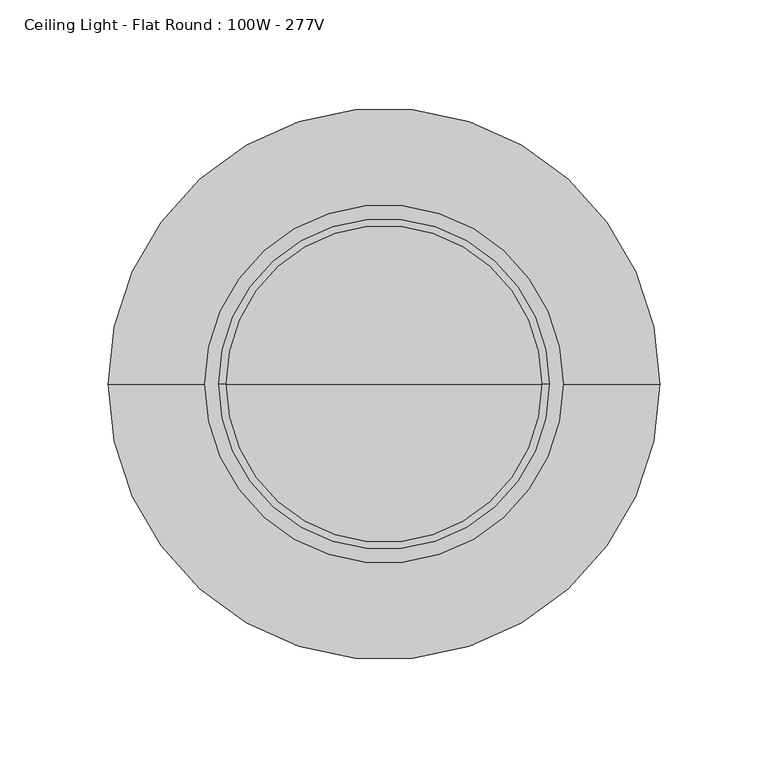
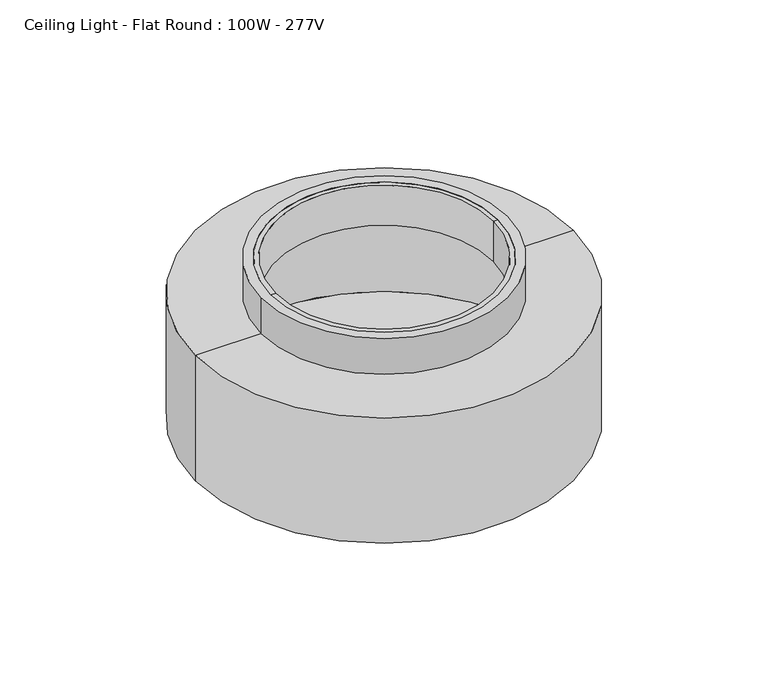
"""IFC4 building model written with IfcOpenShell, lengths in millimetres: light fixture geometry, Ceiling Light - Flat Round : 100W - 277V."""

from ifc_helpers import new_model, si_unit, point, frame, origin, origin_2d, place, context, project, spatial, polyline, circle_curve, trimmed, segment, composite_curve, outline, extrude, source, transform, mapped, element, save
from ifc_brep_helpers import plane_surface, cylinder_surface, revolved_surface, advanced_brep


def ceiling_light_flat_round_100w_277v_0a96185f(model_context):
    return source(origin(), model_context, "Body", "SolidModel", [
        extrude(outline(composite_curve([segment(trimmed(circle_curve(origin_2d(), 82.55), [point((-82.55, 0.0))], [point((82.55, 0.0))], False, "CARTESIAN"), True, "CONTINUOUS"), segment(trimmed(circle_curve(origin_2d(), 82.55), [point((82.55, 0.0))], [point((-82.55, 0.0))], False, "CARTESIAN"), True, "CONTINUOUS")], self_intersect=False), holes=[composite_curve([segment(trimmed(circle_curve(origin_2d(), 76.2), [point((-76.2, 0.0))], [point((76.2, 0.0))], True, "CARTESIAN"), True, "CONTINUOUS"), segment(trimmed(circle_curve(origin_2d(), 76.2), [point((76.2, 0.0))], [point((-76.2, 0.0))], True, "CARTESIAN"), True, "CONTINUOUS")], self_intersect=False)]), frame((0.0, 0.0, 2413.0), z_axis=(0.0, 0.0, 1.0), x_axis=(1.0, 0.0, 0.0)), (0.0, 0.0, 1.0), 25.4),
        advanced_brep(
        [(127.0, 0.0, 2413.0), (-127.0, 0.0, 2413.0), (-76.2, 0.0, 2413.0), (76.2, 0.0, 2413.0), (127.0, 0.0, 2324.1), (-127.0, 0.0, 2324.1), (0.0, 0.0, 2324.1), (123.825, 0.0, 2327.275), (-123.825, 0.0, 2327.275), (0.0, 0.0, 2327.275), (123.825, 0.0, 2409.825), (-123.825, 0.0, 2409.825), (73.025, 0.0, 2409.825), (-73.025, 0.0, 2409.825), (73.025, 0.0, 2438.4), (-73.025, 0.0, 2438.4), (76.2, 0.0, 2438.4), (-76.2, 0.0, 2438.4)],
        [
            (0, 1, circle_curve(frame((0.0, 0.0, 2413.0), z_axis=(0.0, 0.0, 1.0), x_axis=(-1.0, 0.0, 0.0)), 127.0)),
            (1, 2),
            (2, 3, circle_curve(frame((0.0, 0.0, 2413.0), z_axis=(0.0, 0.0, -1.0), x_axis=(-1.0, 0.0, 0.0)), 76.2)),
            (3, 0),
            (1, 0, circle_curve(frame((0.0, 0.0, 2413.0), z_axis=(0.0, 0.0, 1.0), x_axis=(-1.0, 0.0, 0.0)), 127.0)),
            (3, 2, circle_curve(frame((0.0, 0.0, 2413.0), z_axis=(0.0, 0.0, -1.0), x_axis=(-1.0, 0.0, 0.0)), 76.2)),
            (4, 5, circle_curve(frame((0.0, 0.0, 2324.1), z_axis=(0.0, 0.0, 1.0), x_axis=(-1.0, 0.0, 0.0)), 127.0)),
            (5, 1),
            (0, 4),
            (5, 4, circle_curve(frame((0.0, 0.0, 2324.1), z_axis=(0.0, 0.0, 1.0), x_axis=(-1.0, 0.0, 0.0)), 127.0)),
            (6, 5),
            (4, 6),
            (7, 8, circle_curve(frame((0.0, 0.0, 2327.275), z_axis=(0.0, 0.0, 1.0), x_axis=(-1.0, 0.0, 0.0)), 123.825)),
            (8, 9),
            (9, 7),
            (8, 7, circle_curve(frame((0.0, 0.0, 2327.275), z_axis=(0.0, 0.0, 1.0), x_axis=(-1.0, 0.0, 0.0)), 123.825)),
            (10, 11, circle_curve(frame((0.0, 0.0, 2409.825), z_axis=(0.0, 0.0, 1.0), x_axis=(-1.0, 0.0, 0.0)), 123.825)),
            (11, 8),
            (7, 10),
            (11, 10, circle_curve(frame((0.0, 0.0, 2409.825), z_axis=(0.0, 0.0, 1.0), x_axis=(-1.0, 0.0, 0.0)), 123.825)),
            (12, 13, circle_curve(frame((0.0, 0.0, 2409.825), z_axis=(0.0, 0.0, 1.0), x_axis=(-1.0, 0.0, 0.0)), 73.025)),
            (13, 11),
            (10, 12),
            (13, 12, circle_curve(frame((0.0, 0.0, 2409.825), z_axis=(0.0, 0.0, 1.0), x_axis=(-1.0, 0.0, 0.0)), 73.025)),
            (14, 15, circle_curve(frame((0.0, 0.0, 2438.4), z_axis=(0.0, 0.0, 1.0), x_axis=(-1.0, 0.0, 0.0)), 73.025)),
            (15, 13),
            (12, 14),
            (15, 14, circle_curve(frame((0.0, 0.0, 2438.4), z_axis=(0.0, 0.0, 1.0), x_axis=(-1.0, 0.0, 0.0)), 73.025)),
            (16, 17, circle_curve(frame((0.0, 0.0, 2438.4), z_axis=(0.0, 0.0, 1.0), x_axis=(-1.0, 0.0, 0.0)), 76.2)),
            (17, 15),
            (14, 16),
            (17, 16, circle_curve(frame((0.0, 0.0, 2438.4), z_axis=(0.0, 0.0, 1.0), x_axis=(-1.0, 0.0, 0.0)), 76.2)),
            (2, 17),
            (16, 3),
        ],
        [
            plane_surface(frame((0.0, 0.0, 2413.0), z_axis=(0.0, 0.0, 1.0), x_axis=(-1.0, 0.0, 0.0))),
            cylinder_surface(frame((0.0, 0.0, 2463.8), z_axis=(0.0, 0.0, -1.0), x_axis=(-1.0, 0.0, 0.0)), 127.0),
            plane_surface(frame((0.0, 0.0, 2324.1), z_axis=(0.0, 0.0, -1.0), x_axis=(-1.0, 0.0, 0.0))),
            plane_surface(frame((0.0, 0.0, 2327.275), z_axis=(0.0, 0.0, 1.0), x_axis=(-1.0, 0.0, 0.0))),
            revolved_surface(polyline([(-123.825, 0.0, 2327.275), (-123.825, 0.0, 2409.825)]), (0.0, 0.0, 2463.8), (0.0, 0.0, -1.0)),
            plane_surface(frame((0.0, 0.0, 2409.825), z_axis=(0.0, 0.0, -1.0), x_axis=(-1.0, 0.0, 0.0))),
            revolved_surface(polyline([(-73.025, 0.0, 2409.825), (-73.025, 0.0, 2438.4)]), (0.0, 0.0, 2463.8), (0.0, 0.0, -1.0)),
            plane_surface(frame((0.0, 0.0, 2438.4), z_axis=(0.0, 0.0, 1.0), x_axis=(-1.0, 0.0, 0.0))),
            cylinder_surface(frame((0.0, 0.0, 2463.8), z_axis=(0.0, 0.0, -1.0), x_axis=(-1.0, 0.0, 0.0)), 76.2),
        ],
        [
            (0, [[1, 2, 3, 4]]),
            (0, [[5, -4, 6, -2]]),
            (1, [[7, 8, -1, 9]]),
            (1, [[10, -9, -5, -8]]),
            (2, [[11, -7, 12]]),
            (2, [[-12, -10, -11]]),
            (3, [[13, 14, 15]]),
            (3, [[16, -15, -14]]),
            (4, [[17, 18, -13, 19]]),
            (4, [[20, -19, -16, -18]]),
            (5, [[21, 22, -17, 23]]),
            (5, [[24, -23, -20, -22]]),
            (6, [[25, 26, -21, 27]]),
            (6, [[28, -27, -24, -26]]),
            (7, [[29, 30, -25, 31]]),
            (7, [[32, -31, -28, -30]]),
            (8, [[-3, 33, -29, 34]]),
            (8, [[-6, -34, -32, -33]]),
        ],
    ),
    ])


if __name__ == "__main__":
    model = new_model("IFC4")
    model_context = context("Model", 3, world=origin())
    ifc_project = project(units=[si_unit("LENGTHUNIT", "METRE", prefix="MILLI")], contexts=[model_context])
    site = spatial("IfcSite", under=ifc_project)
    building = spatial("IfcBuilding", under=site)
    placement = place(None, origin())
    ceiling_light_flat_round_100w_277v_shape = ceiling_light_flat_round_100w_277v_0a96185f(model_context)
    element("IfcLightFixture", 1, ObjectType="Ceiling Light - Flat Round : 100W - 277V", at=placement, inside=building, context=model_context, shape_type="MappedRepresentation", body=[
        mapped(ceiling_light_flat_round_100w_277v_shape, transform((0.0, 0.0, 0.0), x_axis=(1.0, 0.0, 0.0), y_axis=(0.0, 1.0, 0.0), z_axis=(0.0, 0.0, 1.0))),
    ])
    save(model, "model.ifc")

# Revit data of these elements
# Type "Ceiling Light - Flat Round : 100W - 277V"
#   Lamp = "A-19"
#   Assembly Code = "D5020220"
#   Wattage = 100 W
#   built-in parameter 1150110 = 1 (stored number, unit not read)
#   built-in parameter 1114217 = 1 (stored number, unit not read)
#   built-in parameter 1150109 = 1 (stored number, unit not read)
#   built-in parameter 1150113 = 1 (stored number, unit not read)
#   built-in parameter 1150115 = 1 (stored number, unit not read)
#   built-in parameter 1150105 = 557.042 (stored number, unit not read)
#   Light Source Symbol Size = 2' - 0"
#   built-in parameter 1150112 = 1 (stored number, unit not read)
#   built-in parameter 1150114 = 1 (stored number, unit not read)
#   built-in parameter 1150107 = 2800 (stored number, unit not read)
#   built-in parameter 1150106 = 5.57042 (stored number, unit not read)
#   Emit from Circle Diameter = 0' - 10"
#   built-in parameter 1150104 = 1.6258 (stored number, unit not read)
#   Ballast Voltage = 277 V
#   built-in parameter 1114218 = 1 (stored number, unit not read)
#   built-in parameter 1150133 = 10 (stored number, unit not read)
#   Lumens = 1750 lm
#   Apparent Load = 100 VA
#   built-in parameter 1150134 = 4
#   built-in parameter 1150137 = 1
#   Color Filter = 16777215
#   built-in parameter 1140040 [instance default] = 1
#   Ballast Number of Poles = 1
#   Light Box Material = Steel, Paint Finish, Dark Gray, Matte
#   Diffuser Material = Glass, White, High Luminance
#   Wattage Comments = ""
#   Emit Shape Visible in Rendering = no
#   Dimming Lamp Color Temperature Shift = (empty or 0)
#   Default Elevation = 0
# Element 1 (IfcLightFixture, "Ceiling Light - Flat Round : 100W - 277V")
#   Materials on its faces: "Glass, White, High Luminance", "Steel, Paint Finish, Dark Gray, Matte"
# Materials
#   "Steel, Paint Finish, Dark Gray, Matte": class "Metal", colour RGB 98 98 98, transparency 0, Description = "Steel, paint finish, dark gray, matte", Cost = 0
#   "Glass, White, High Luminance": class "Glass", colour RGB 249 250 249, transparency 0.8, Description = "physical material", Cost = 0
